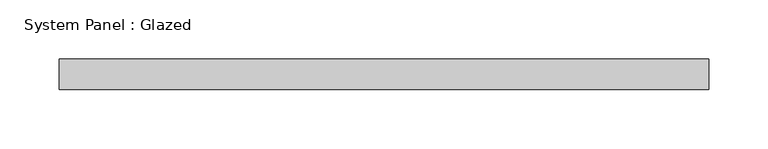
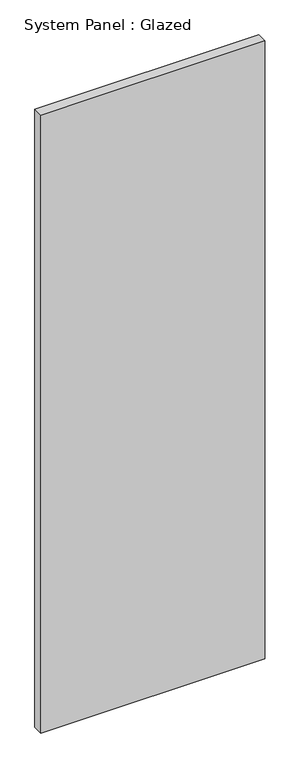
"""IFC4 building model written with IfcOpenShell, lengths in millimetres: plate geometry, System Panel : Glazed."""

from ifc_helpers import new_model, si_unit, origin, origin_with_axes, place, context, project, spatial, polyline, outline, extrude, source, transform, mapped, element, save


def system_panel_glazed_66fd639c(model_context):
    return source(origin(), model_context, "Body", "SweptSolid", [
        extrude(outline(polyline([(273.05, 19.05), (-273.05, 19.05), (-273.05, 44.45), (273.05, 44.45), (273.05, 19.05)])), origin_with_axes(), (0.0, 0.0, 1.0), 1593.7849865),
    ])


if __name__ == "__main__":
    model = new_model("IFC4")
    model_context = context("Model", 3, world=origin())
    ifc_project = project(units=[si_unit("LENGTHUNIT", "METRE", prefix="MILLI")], contexts=[model_context])
    site = spatial("IfcSite", under=ifc_project)
    building = spatial("IfcBuilding", under=site)
    placement = place(None, origin())
    system_panel_glazed_shape = system_panel_glazed_66fd639c(model_context)
    element("IfcPlate", 1, ObjectType="System Panel : Glazed", at=placement, inside=building, context=model_context, shape_type="MappedRepresentation", body=[
        mapped(system_panel_glazed_shape, transform((0.0, 0.0, 0.0), x_axis=(1.0, 0.0, 0.0), y_axis=(0.0, 1.0, 0.0), z_axis=(0.0, 0.0, 1.0))),
    ])
    save(model, "model.ifc")

# Revit data of these elements
# Type "System Panel : Glazed"
#   Construction Type Id = "GSP4R"
#   Analytic Construction = "1/8 in Pilkington single glazing"
#   Visual Light Transmittance = 0.9
#   Solar Heat Gain Coefficient = 0.86
#   Heat Transfer Coefficient (U) = 1.18115 BTU/(h·ft²·°F)
#   Define Thermal Properties by = 1
# Element 1 (IfcPlate, "System Panel : Glazed")
#   Materials on its faces: "Glass"
# Materials
#   "Glass": class "Glass", colour RGB 0 128 192, transparency 0.75, Description = "Soda Lime Glass", Cost = 0
